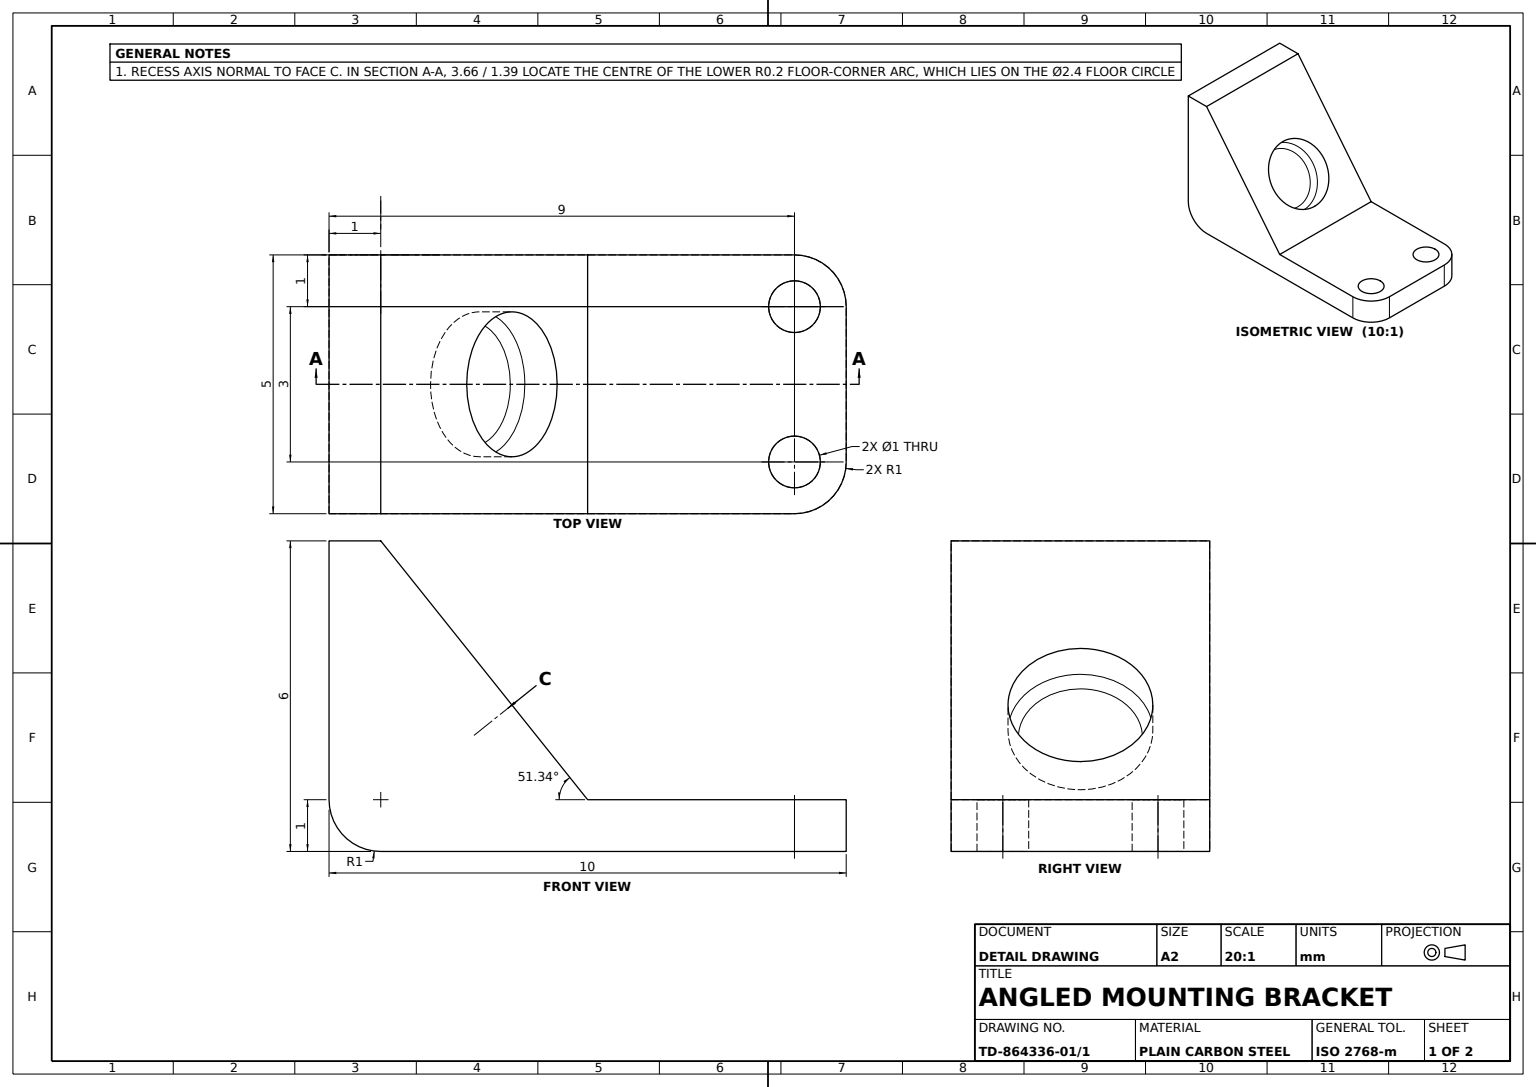
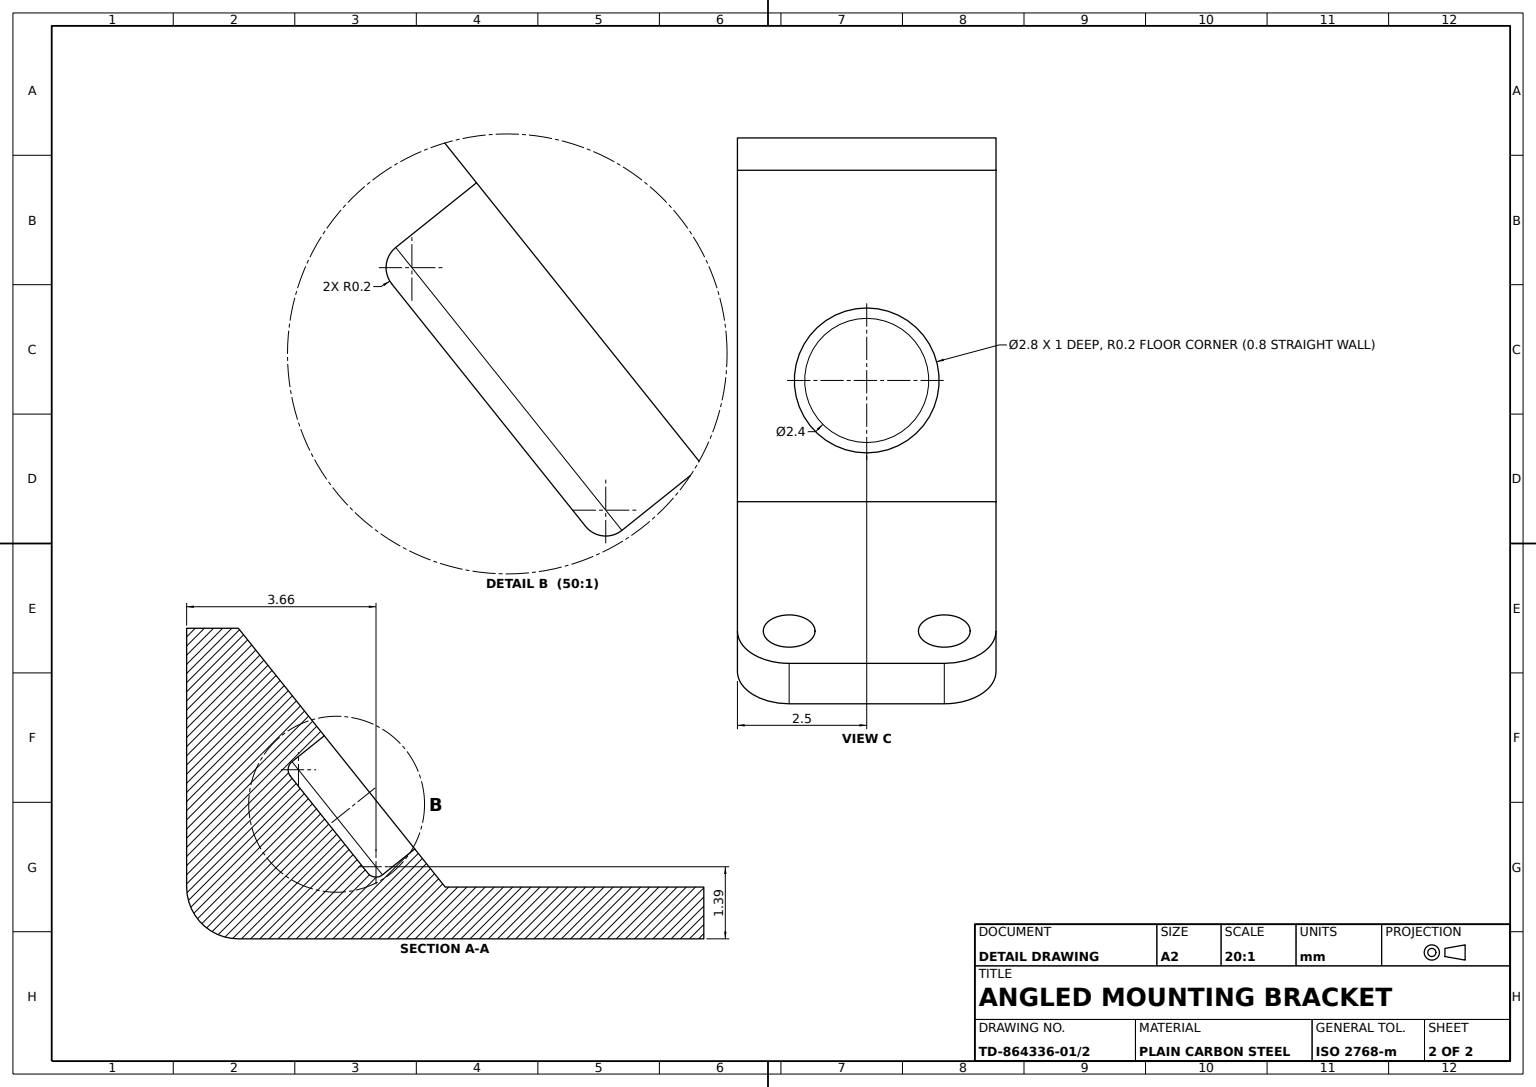
SolidWorks part; units mm, degrees
material "Plain Carbon Steel"
ref_plane "Front Plane" through (0, 0, 0) normal (0, 0, 1) x (1, 0, 0)
ref_plane "Top Plane" through (0, 0, 0) normal (0, 1, 0) x (1, 0, 0)
ref_plane "Right Plane" through (0, 0, 0) normal (1, 0, 0) x (0, 0, -1)
sketch "Bracket Profile Sketch" plane through (0, 0, 0) normal (0, 0, 1) x (1, 0, 0)
  line L0 (0, 1) -> (0, 6)
  line L1 (0, 6) -> (1, 6)
  line L2 (1, 6) -> (5, 1)
  line L3 (5, 1) -> (10, 1)
  line L4 (10, 1) -> (10, 0)
  line L5 (10, 0) -> (1, 0)
  arc A0 (0, 1) -> (1, 0) centre (1, 1) ccw
  point P9 (0, 0)
  dimension "D5" = 1
  dimension "D1" = 6
  dimension "D2" = 1
  dimension "D3" = 10
  dimension "D4" = 5
  dimension "D6" = 1
extrude "Bracket Body" add sketch "Bracket Profile Sketch" along normal mid plane 5
sketch "Face Recess Sketch" plane through (3.5366, 2.8293, 0) normal (0.7809, 0.6247, 0) x (0, 0, -1)
  circle A0 centre (0, 0) radius 1.4
  dimension "D1" = 2.8
extrude "Face Recess Ø2.8x1" cut sketch "Face Recess Sketch" against normal blind 1
sketch "Mounting Holes Sketch" plane through (0, 1, 0) normal (0, 1, 0) x (1, 0, 0)
  line L0 (5, -2.5) -> (5, 2.5) construction
  line L1 (0, 0) -> (12.4679, 0) construction
  circle A0 centre (9, -1.5) radius 0.5
  circle A1 centre (9, 1.5) radius 0.5
  dimension "D2" = 1
  dimension "D3" = 1
  dimension "D1" = 4
  dimension "D4" = 1.5
extrude "Foot Mounting Holes" cut sketch "Mounting Holes Sketch" against normal through all
fillet "Corner Fillets R1" radius 1 2 edges at (10, 0.5, 2.5) (10, 0.5, -2.5)
fillet "Recess Edge Fillet R0.2" radius 0.2 1 edges at (1.8811, 3.2978, 0)
